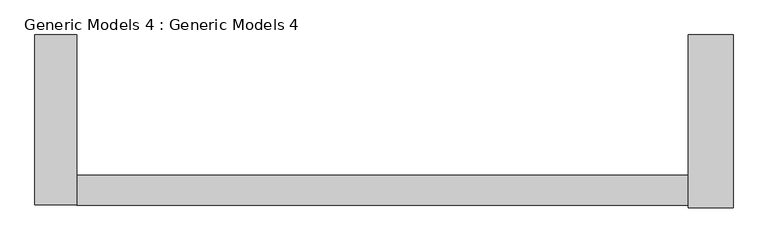
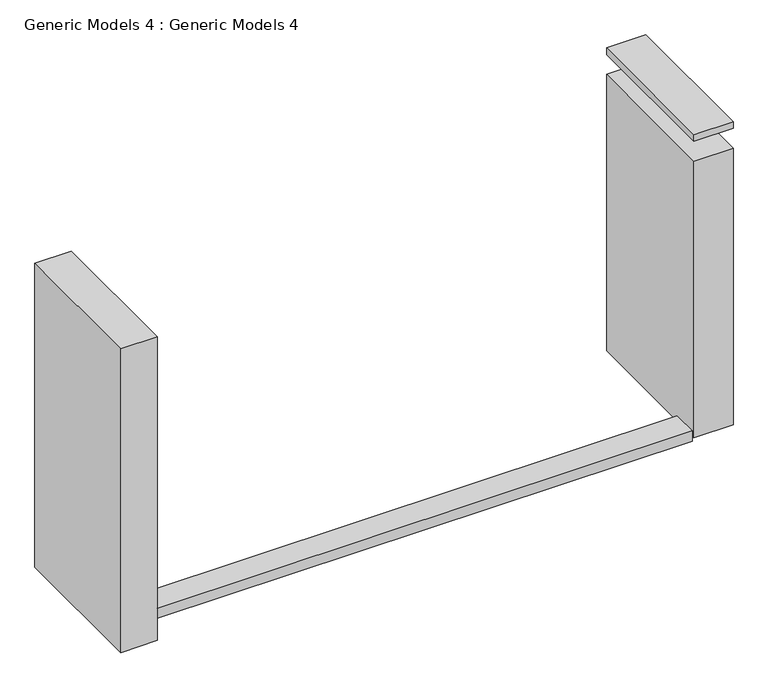
"""IFC4 building model written with IfcOpenShell, lengths in millimetres: proxy geometry, Generic Models 4 : Generic Models 4."""

from ifc_helpers import new_model, si_unit, frame, origin, origin_with_axes, place, context, project, spatial, polyline, outline, extrude, source, transform, mapped, element, save


def generic_models_4_generic_models_4_71681450(model_context):
    return source(origin(), model_context, "Body", "SweptSolid", [
        extrude(outline(polyline([(-10534.5831929, -10286.4592534), (-10178.9831929, -10286.4592534), (-10178.9831929, -11734.2592534), (-10534.5831929, -11734.2592534), (-10534.5831929, -10286.4592534)])), frame((0.0, 0.0, -279.4), z_axis=(0.0, 0.0, 1.0), x_axis=(1.0, 0.0, 0.0)), (0.0, 0.0, 1.0), 3124.8571484),
        extrude(outline(polyline([(-10178.9831929, -11480.2592534), (-4971.9831929, -11480.2592534), (-4971.9831929, -11734.2592534), (-10178.9831929, -11734.2592534), (-10178.9831929, -11480.2592534)])), frame((0.0, 0.0, -50.8), z_axis=(0.0, 0.0, 1.0), x_axis=(1.0, 0.0, 0.0)), (0.0, 0.0, 1.0), 104.303275),
        extrude(outline(polyline([(-4971.9831929, -10286.4592534), (-4590.9831929, -10286.4592534), (-4590.9831929, -11759.6592534), (-4971.9831929, -11759.6592534), (-4971.9831929, -10286.4592534)])), frame((0.0, 0.0, 3048.0), z_axis=(0.0, 0.0, 1.0), x_axis=(1.0, 0.0, 0.0)), (0.0, 0.0, 1.0), 68.296843),
        extrude(outline(polyline([(-4590.9831929, -10286.4592534), (-4590.9831929, -11759.6592534), (-4971.9831929, -11759.6592534), (-4971.9831929, -10286.4592534), (-4590.9831929, -10286.4592534)])), origin_with_axes(), (0.0, 0.0, 1.0), 2845.4571484),
    ])


if __name__ == "__main__":
    model = new_model("IFC4")
    model_context = context("Model", 3, world=origin())
    ifc_project = project(units=[si_unit("LENGTHUNIT", "METRE", prefix="MILLI")], contexts=[model_context])
    site = spatial("IfcSite", under=ifc_project)
    building = spatial("IfcBuilding", under=site)
    placement = place(None, origin())
    generic_models_4_generic_models_4_shape = generic_models_4_generic_models_4_71681450(model_context)
    element("IfcBuildingElementProxy", 1, Name="Generic Models 4 : Generic Models 4", ObjectType="Generic Models 4 : Generic Models 4", at=placement, inside=building, context=model_context, shape_type="MappedRepresentation", body=[
        mapped(generic_models_4_generic_models_4_shape, transform((0.0, 0.0, 0.0), x_axis=(1.0, 0.0, 0.0), y_axis=(0.0, 1.0, 0.0), z_axis=(0.0, 0.0, 1.0))),
    ])
    save(model, "model.ifc")

# Revit data of these elements
# Element 1 (IfcBuildingElementProxy, "Generic Models 4 : Generic Models 4")
#   Materials on its faces: "Tile, Porcelain, 4in"
# Materials
#   "Tile, Porcelain, 4in": class "Generic", colour RGB 89 87 158, transparency 0, Description = "Porcelain tile, 4\", white", Cost = 0
